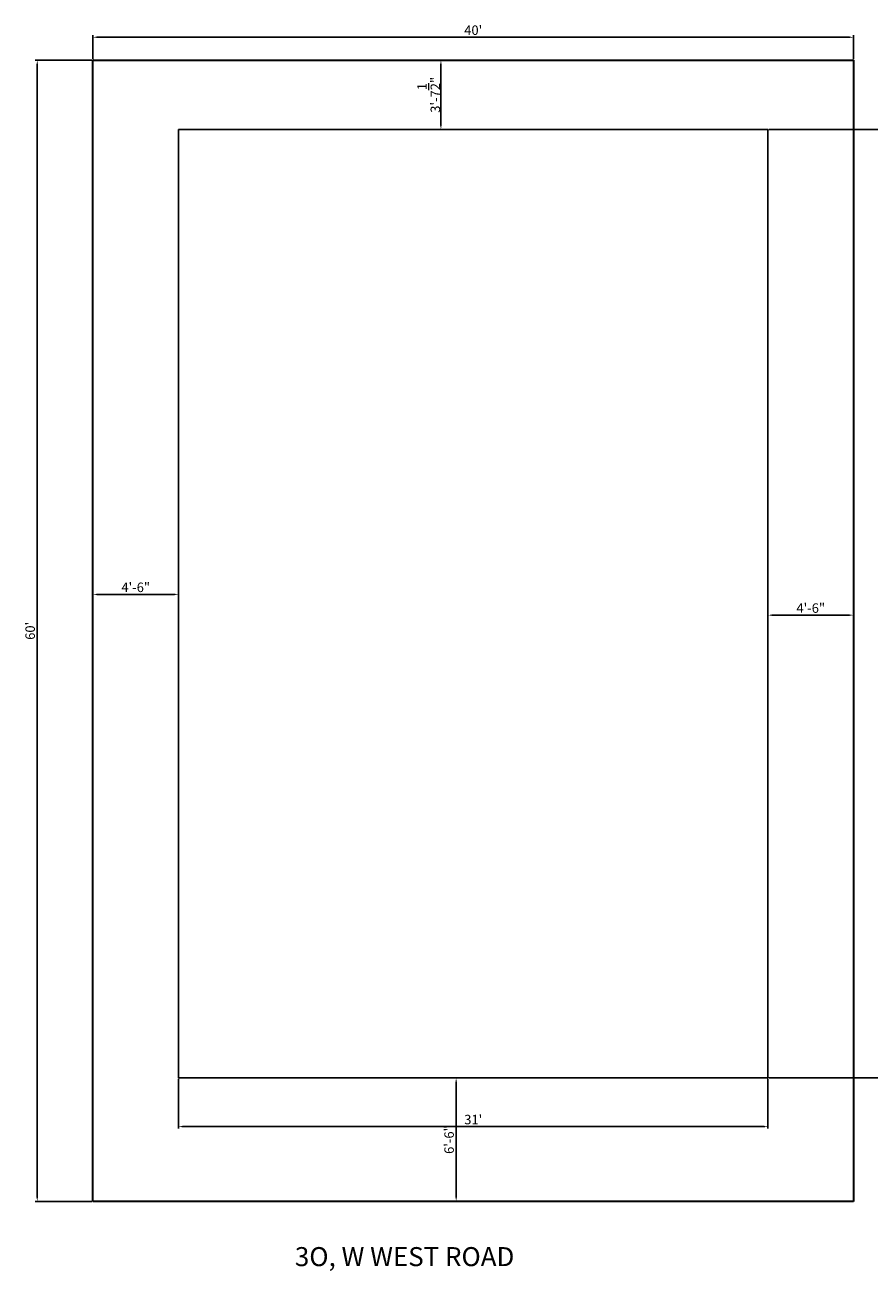
# Model space of a CAD drawing. Units: inches. Extents: x 1678 to 4856, y 4 to 3876.
# Tile 1 of 4: x 1678 to 2211, y 3064 to 3851. Entities that reach past the tile are written whole.
import ezdxf

# ---------------------------------------------------------------- set-up
doc = ezdxf.new("R2010")
doc.units = ezdxf.units.IN
for name, color, linetype, lineweight in [('A-ANNO-TEXT', 7, 'Continuous', 18), ('C-BLDG', 7, 'Continuous', 25), ('compound wall', 7, 'Continuous', 30), ('DIMENSIONS', 6, 'Continuous', 18)]:
    doc.layers.add(name, color=color, linetype=linetype, lineweight=lineweight)
doc.styles.get("Standard").update_dxf_attribs({"font": 'arial.ttf'})
doc.dimstyles.new('ISO-25', dxfattribs={"dimtxt": 6, "dimasz": 2.5, "dimexe": 1.25, "dimexo": 0.625, "dimtad": 1, "dimdec": 1, "dimlunit": 4, "dimtxsty": 'Standard', "dimcen": 2.5, "dimadec": 0, "dimazin": 0, "dimtfac": 1, "dimtdec": 1, "dimtmove": 0, "dimatfit": 3, "dimfxl": 1, "dimarcsym": 0})

# ---------------------------------------------------------------- blocks, each defined once
blk = doc.blocks.new('*D6')
at = {"layer": 'Defpoints', "color": 0, "transparency": 16777216}
for p in [(1945.98, 3828.28), (1940.38, 3784.66), (1945.98, 3784.66)]:
    blk.add_point(p, dxfattribs=at)
at = {"layer": 'DIMENSIONS', "color": 0, "lineweight": -2, "transparency": 16777216}
for p, q in [((1945.36, 3828.28), (1939.13, 3828.28)), ((1940.38, 3825.78), (1940.38, 3787.16)), ((1945.36, 3784.66), (1939.13, 3784.66))]:
    blk.add_line(p, q, dxfattribs=at)
at = {"layer": 'DIMENSIONS', "color": 0, "transparency": 16777216}
for points in [[(1939.97, 3825.78), (1940.8, 3825.78), (1940.38, 3828.28)], [(1939.97, 3787.16), (1940.8, 3787.16), (1940.38, 3784.66)]]:
    blk.add_solid(points, dxfattribs=at)
at = {"layer": 'DIMENSIONS', "color": 0, "transparency": 16777216, "insert": (1932.68, 3806.47), "char_height": 6, "attachment_point": 5, "rotation": 90}
blk.add_mtext('3\'-7{\\H1x;\\S1/2;}"', dxfattribs=at)
blk = doc.blocks.new('*D7')
at = {"layer": 'Defpoints', "color": 0, "transparency": 16777216}
for p in [(1774.78, 3491.28), (1720.78, 3484.87), (1774.78, 3484.87)]:
    blk.add_point(p, dxfattribs=at)
at = {"layer": 'DIMENSIONS', "color": 0, "lineweight": -2, "transparency": 16777216}
for p, q in [((1720.78, 3485.5), (1720.78, 3492.53)), ((1723.28, 3491.28), (1772.28, 3491.28)), ((1774.78, 3485.5), (1774.78, 3492.53))]:
    blk.add_line(p, q, dxfattribs=at)
at = {"layer": 'DIMENSIONS', "color": 0, "transparency": 16777216}
for points in [[(1723.28, 3491.69), (1723.28, 3490.86), (1720.78, 3491.28)], [(1772.28, 3491.69), (1772.28, 3490.86), (1774.78, 3491.28)]]:
    blk.add_solid(points, dxfattribs=at)
at = {"layer": 'DIMENSIONS', "color": 0, "transparency": 16777216, "insert": (1747.78, 3494.96), "char_height": 6, "attachment_point": 5}
blk.add_mtext('4\'-6"', dxfattribs=at)
blk = doc.blocks.new('*D8')
at = {"layer": 'Defpoints', "color": 0, "transparency": 16777216}
for p in [(2146.78, 3477.37), (2200.78, 3478.17), (2200.78, 3477.37)]:
    blk.add_point(p, dxfattribs=at)
at = {"layer": 'DIMENSIONS', "color": 0, "lineweight": -2, "transparency": 16777216}
for p, q in [((2146.78, 3477.99), (2146.78, 3479.42)), ((2149.28, 3478.17), (2198.28, 3478.17)), ((2200.78, 3477.99), (2200.78, 3479.42))]:
    blk.add_line(p, q, dxfattribs=at)
at = {"layer": 'DIMENSIONS', "color": 0, "transparency": 16777216}
for points in [[(2149.28, 3478.59), (2149.28, 3477.75), (2146.78, 3478.17)], [(2198.28, 3478.59), (2198.28, 3477.75), (2200.78, 3478.17)]]:
    blk.add_solid(points, dxfattribs=at)
at = {"layer": 'DIMENSIONS', "color": 0, "transparency": 16777216, "insert": (2173.78, 3481.86), "char_height": 6, "attachment_point": 5}
blk.add_mtext('4\'-6"', dxfattribs=at)
blk = doc.blocks.new('*D9')
at = {"layer": 'Defpoints', "color": 0, "transparency": 16777216}
for p in [(1960.78, 3186.28), (1950, 3108.28), (1960.78, 3108.28)]:
    blk.add_point(p, dxfattribs=at)
at = {"layer": 'DIMENSIONS', "color": 0, "lineweight": -2, "transparency": 16777216}
for p, q in [((1960.16, 3186.28), (1948.75, 3186.28)), ((1950, 3183.78), (1950, 3110.78)), ((1960.16, 3108.28), (1948.75, 3108.28))]:
    blk.add_line(p, q, dxfattribs=at)
at = {"layer": 'DIMENSIONS', "color": 0, "transparency": 16777216}
for points in [[(1949.58, 3183.78), (1950.41, 3183.78), (1950, 3186.28)], [(1949.58, 3110.78), (1950.41, 3110.78), (1950, 3108.28)]]:
    blk.add_solid(points, dxfattribs=at)
at = {"layer": 'DIMENSIONS', "color": 0, "transparency": 16777216, "insert": (1946.31, 3147.28), "char_height": 6, "attachment_point": 5, "rotation": 90}
blk.add_mtext('6\'-6"', dxfattribs=at)
blk = doc.blocks.new('*D13')
at = {"layer": 'Defpoints', "color": 0, "transparency": 16777216}
for p in [(2200.78, 3842.8), (1720.78, 3828.28), (2200.78, 3828.28)]:
    blk.add_point(p, dxfattribs=at)
at = {"layer": 'DIMENSIONS', "color": 0, "lineweight": -2, "transparency": 16777216}
for p, q in [((1720.78, 3828.9), (1720.78, 3844.05)), ((1723.28, 3842.8), (2198.28, 3842.8)), ((2200.78, 3828.9), (2200.78, 3844.05))]:
    blk.add_line(p, q, dxfattribs=at)
at = {"layer": 'DIMENSIONS', "color": 0, "transparency": 16777216}
for points in [[(1723.28, 3843.21), (1723.28, 3842.38), (1720.78, 3842.8)], [(2198.28, 3843.21), (2198.28, 3842.38), (2200.78, 3842.8)]]:
    blk.add_solid(points, dxfattribs=at)
at = {"layer": 'DIMENSIONS', "color": 0, "transparency": 16777216, "insert": (1960.78, 3846.48), "char_height": 6, "attachment_point": 5}
blk.add_mtext("40'", dxfattribs=at)
blk = doc.blocks.new('*D14')
at = {"layer": 'Defpoints', "color": 0, "transparency": 16777216}
for p in [(1720.78, 3828.28), (1685.63, 3108.28), (1720.78, 3108.28)]:
    blk.add_point(p, dxfattribs=at)
at = {"layer": 'DIMENSIONS', "color": 0, "lineweight": -2, "transparency": 16777216}
for p, q in [((1720.16, 3828.28), (1684.38, 3828.28)), ((1685.63, 3825.78), (1685.63, 3110.78)), ((1720.16, 3108.28), (1684.38, 3108.28))]:
    blk.add_line(p, q, dxfattribs=at)
at = {"layer": 'DIMENSIONS', "color": 0, "transparency": 16777216}
for points in [[(1685.22, 3825.78), (1686.05, 3825.78), (1685.63, 3828.28)], [(1685.22, 3110.78), (1686.05, 3110.78), (1685.63, 3108.28)]]:
    blk.add_solid(points, dxfattribs=at)
at = {"layer": 'DIMENSIONS', "color": 0, "transparency": 16777216, "insert": (1681.94, 3468.28), "char_height": 6, "attachment_point": 5, "rotation": 90}
blk.add_mtext("60'", dxfattribs=at)
blk = doc.blocks.new('*D15')
at = {"layer": 'Defpoints', "color": 0, "transparency": 16777216}
for p in [(1774.78, 3186.28), (2146.78, 3186.28), (2146.78, 3155.44)]:
    blk.add_point(p, dxfattribs=at)
at = {"layer": 'DIMENSIONS', "color": 0, "lineweight": -2, "transparency": 16777216}
for p, q in [((1774.78, 3185.65), (1774.78, 3154.19)), ((2146.78, 3185.65), (2146.78, 3154.19)), ((1777.28, 3155.44), (2144.28, 3155.44))]:
    blk.add_line(p, q, dxfattribs=at)
at = {"layer": 'DIMENSIONS', "color": 0, "transparency": 16777216}
for points in [[(1777.28, 3155.85), (1777.28, 3155.02), (1774.78, 3155.44)], [(2144.28, 3155.85), (2144.28, 3155.02), (2146.78, 3155.44)]]:
    blk.add_solid(points, dxfattribs=at)
at = {"layer": 'DIMENSIONS', "color": 0, "transparency": 16777216, "insert": (1960.78, 3159.13), "char_height": 6, "attachment_point": 5}
blk.add_mtext("31'", dxfattribs=at)
blk = doc.blocks.new('SITE-PERIMETER-40x60')
for p, q in [((0, 720), (480, 720)), ((0, 0), (0, 720)), ((480, 720), (480, 0)), ((480, 0), (0, 0))]:
    blk.add_line(p, q)
blk = doc.blocks.new('*D56')
at = {"layer": 'Defpoints', "color": 0, "transparency": 16777216}
for p in [(2146.78, 3784.66), (2240.93, 3784.66), (2146.78, 3186.28)]:
    blk.add_point(p, dxfattribs=at)
at = {"layer": 'DIMENSIONS', "color": 0, "lineweight": -2, "transparency": 16777216}
for p, q in [((2147.41, 3784.66), (2242.18, 3784.66)), ((2240.93, 3188.78), (2240.93, 3782.16)), ((2147.41, 3186.28), (2242.18, 3186.28))]:
    blk.add_line(p, q, dxfattribs=at)
at = {"layer": 'DIMENSIONS', "color": 0, "transparency": 16777216}
for points in [[(2240.52, 3782.16), (2241.35, 3782.16), (2240.93, 3784.66)], [(2240.52, 3188.78), (2241.35, 3188.78), (2240.93, 3186.28)]]:
    blk.add_solid(points, dxfattribs=at)
at = {"layer": 'DIMENSIONS', "color": 0, "transparency": 16777216, "insert": (2237.2, 3485.47), "char_height": 6, "attachment_point": 5, "rotation": 90}
blk.add_mtext('49\'-10 1/2"', dxfattribs=at)

msp = doc.modelspace()

# ---------------------------------------------------------------- linework, layer by layer
at = {"layer": 'C-BLDG'}
for p, q in [((1774.78, 3784.66), (2146.78, 3784.66)), ((1774.78, 3186.28), (1774.78, 3784.66)), ((2146.78, 3784.66), (2146.78, 3186.28)), ((2146.78, 3186.28), (1774.78, 3186.28))]:
    msp.add_line(p, q, dxfattribs=at)

# ---------------------------------------------------------------- block references
at = {"layer": 'compound wall'}
msp.add_blockref('SITE-PERIMETER-40x60', (1720.78, 3108.28), dxfattribs=at)

# ---------------------------------------------------------------- texts
at = {"layer": 'A-ANNO-TEXT', "insert": (1848.24, 3079.43), "char_height": 12, "attachment_point": 1}
msp.add_mtext_dynamic_manual_height_columns('3O, W WEST ROAD ', width=221.8792, gutter_width=12.5, heights=[0], dxfattribs=at)

# ---------------------------------------------------------------- dimensions: what is measured, and where the dimension line sits
at = {"layer": 'DIMENSIONS'}
for base, p1, p2, picture, middle in [((2200.78, 3842.8), (1720.78, 3828.28), (2200.78, 3828.28), '*D13', (1960.78, 3846.48)), ((1774.78, 3491.28), (1720.78, 3484.87), (1774.78, 3484.87), '*D7', (1747.78, 3494.96)), ((2200.78, 3478.17), (2146.78, 3477.37), (2200.78, 3477.37), '*D8', (2173.78, 3481.86)), ((2146.78, 3155.44), (1774.78, 3186.28), (2146.78, 3186.28), '*D15', (1960.78, 3159.13))]:
    dim = msp.add_linear_dim(base=base, p1=p1, p2=p2, dimstyle='ISO-25', override={"dimclrd": 0, "dimclre": 0, "dimclrt": 0}, dxfattribs=at)
    dim.commit()
    dim.dimension.update_dxf_attribs({"geometry": picture, "text_midpoint": middle})
for base, p1, p2, override, picture, middle in [((1685.63, 3108.28), (1720.78, 3828.28), (1720.78, 3108.28), {"dimclrd": 0, "dimclre": 0, "dimclrt": 0}, '*D14', (1681.94, 3468.28)), ((1940.38, 3784.66), (1945.98, 3828.28), (1945.98, 3784.66), {"dimclrd": 0, "dimclre": 0, "dimclrt": 0}, '*D6', (1932.68, 3806.47)), ((2240.93, 3784.66), (2146.78, 3186.28), (2146.78, 3784.66), {"dimdec": 1, "dimlfac": 1, "dimrnd": 0, "dimzin": 1, "dimdsep": 46, "dimlunit": 4, "dimfrac": 2}, '*D56', (2237.2, 3485.47)), ((1950, 3108.28), (1960.78, 3186.28), (1960.78, 3108.28), {"dimclrd": 0, "dimclre": 0, "dimclrt": 0}, '*D9', (1946.31, 3147.28))]:
    dim = msp.add_linear_dim(base=base, p1=p1, p2=p2, angle=90, dimstyle='ISO-25', override=override, dxfattribs=at)
    dim.commit()
    dim.dimension.update_dxf_attribs({"geometry": picture, "text_midpoint": middle})

doc.saveas('drawing.dxf')
